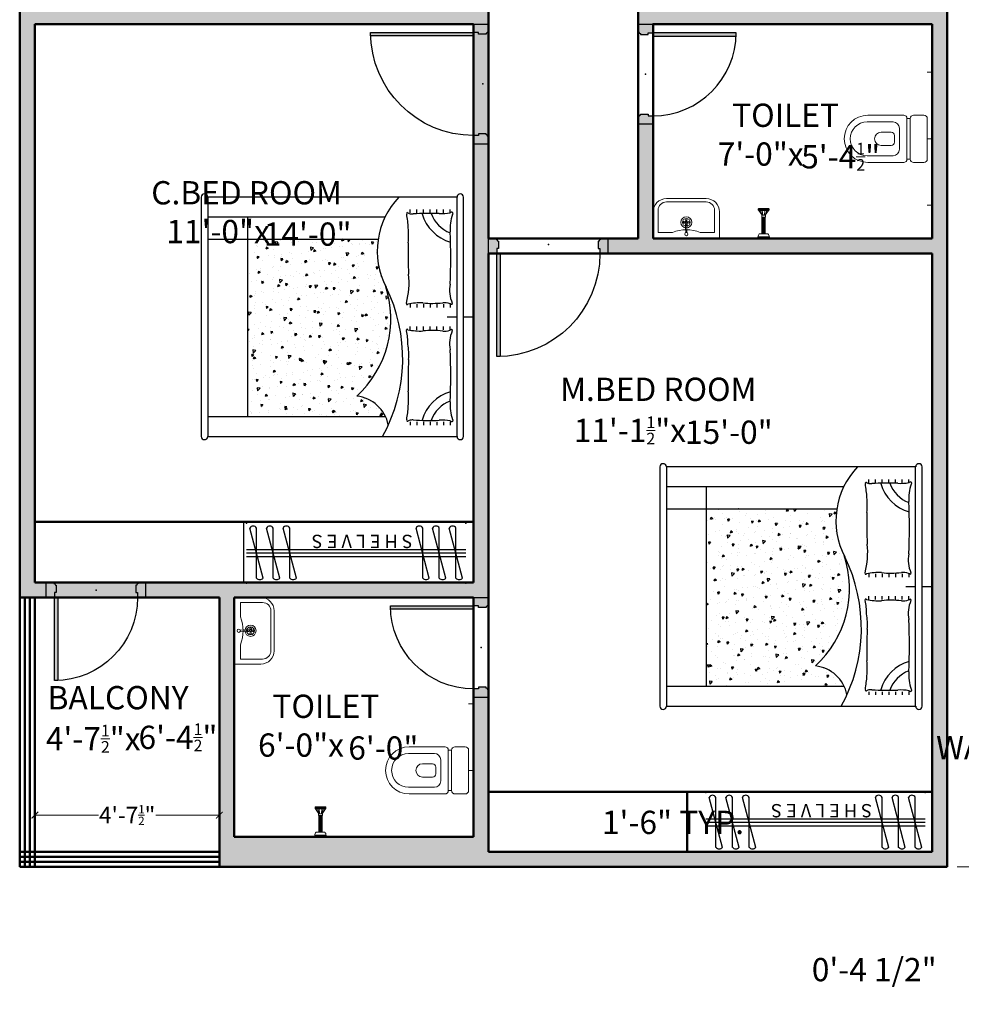
# Model space of a CAD drawing. Units: inches. Extents: x 4508 to 5907, y 877 to 1592.
# Tile 2 of 20: x 4919 to 5203, y 885 to 1182. Entities that reach past the tile are written whole.
import ezdxf

# ---------------------------------------------------------------- set-up
doc = ezdxf.new("R2010")
doc.units = ezdxf.units.IN
doc.layers.get('DEFPOINTS').update_dxf_attribs({"color": 8})
for name, color, linetype, lineweight in [('A-ANNO-DIMS', 2, 'Continuous', 18), ('A-DOOR', 4, 'Continuous', 25), ('A-FLOR-CASE', 30, 'Continuous', 25), ('A-FLOR-FIXT', 8, 'Continuous', 18), ('A-FURN', 24, 'Continuous', 18), ('A-WALL', 7, 'Continuous', 50), ('A-WALL-PATT', 8, 'Continuous', 13)]:
    doc.layers.add(name, color=color, linetype=linetype, lineweight=lineweight)
doc.layers.add('doors & windows', color=30, linetype='Continuous')
doc.layers.add('furniture', color=24, linetype='Continuous')
doc.styles.get("Standard").update_dxf_attribs({"font": 'arial.ttf'})
doc.dimstyles.new('details', dxfattribs={"dimtxt": 5, "dimasz": 2, "dimexe": 2, "dimexo": 3, "dimgap": 1, "dimtad": 0, "dimdec": 1, "dimzin": 0, "dimdsep": 46, "dimlunit": 4, "dimtxsty": 'Standard', "dimblk": 'ARCHTICK', "dimcen": 3, "dimclrd": 256, "dimclre": 256, "dimclrt": 256, "dimadec": 0, "dimazin": 0, "dimtfac": 0.5, "dimtdec": 1, "dimtofl": 0, "dimtmove": 0, "dimatfit": 3, "dimldrblk": 'CLOSEDBLANK', "dimfxl": 2, "dimtolj": 1, "dimtzin": 0, "dimlwd": -1, "dimlwe": -1, "dimarcsym": 0})
doc.dimstyles.new('text', dxfattribs={"dimtxt": 7, "dimasz": 0, "dimexe": 3, "dimexo": 3, "dimgap": 0, "dimtad": 1, "dimtih": 1, "dimtoh": 1, "dimzin": 3, "dimdsep": 46, "dimlunit": 4, "dimtxsty": 'Standard', "dimblk": 'CLOSEDBLANK', "dimcen": 3, "dimse1": 1, "dimse2": 1, "dimsd1": 1, "dimsd2": 1, "dimclrd": 256, "dimclre": 256, "dimclrt": 256, "dimadec": 0, "dimazin": 0, "dimtfac": 0.5, "dimtofl": 0, "dimtmove": 0, "dimatfit": 3, "dimfxl": 3, "dimtolj": 1, "dimtzin": 0, "dimlwd": -1, "dimlwe": -1, "dimarcsym": 0})

# ---------------------------------------------------------------- blocks, each defined once
blk = doc.blocks.new('D2')
at = {"layer": 'doors & windows'}
h = blk.add_hatch(dxfattribs=at)
h.set_pattern_fill('DOTS', color=256, scale=2, angle=180, style=0)
h.set_pattern_definition([(180, (0, -4), (-0.0625, -0.125), [0, -0.125])])
h.paths.add_polyline_path([(2.5, 0), (3.5, 0), (3.5, 24.98, 0.010003), (2.5, 25)])
h = blk.add_hatch(dxfattribs=at)
h.set_pattern_fill('DOTS', color=256, scale=2, angle=180, style=0)
h.set_pattern_definition([(180, (0, 0), (-0.0625, -0.125), [0, -0.125])])
edge = h.paths.add_edge_path()
edge.add_line((27.5, 0), (27.5, -1.5))
edge.add_line((27.5, -1.5), (27, -1.5))
edge.add_line((27, -1.5), (27, -3.75))
edge.add_line((27, -3.75), (27.25, -3.75))
edge.add_arc((27.76, -3.74), 0.509, 181.0059, 268.9941)
edge.add_line((27.75, -4.25), (27.75, -4.5))
edge.add_line((27.75, -4.5), (30, -4.5))
edge.add_line((30, -4.5), (30, 0))
edge.add_line((30, 0), (27.5, 0))
edge = h.paths.add_edge_path()
edge.add_line((2.5, -1.5), (2.5, 0))
edge.add_line((2.5, 0), (0, 0))
edge.add_line((0, 0), (0, -4.5))
edge.add_line((0, -4.5), (2.25, -4.5))
edge.add_line((2.25, -4.5), (2.25, -4.25))
edge.add_arc((2.24, -3.74), 0.509, 271.0059, 358.9941)
edge.add_line((2.75, -3.75), (3, -3.75))
edge.add_line((3, -3.75), (3, -1.5))
edge.add_line((3, -1.5), (2.5, -1.5))
for p, q in [((0, 0), (0, -4.5)), ((30, 0), (30, -4.5))]:
    blk.add_line(p, q)
blk.add_lwpolyline([(3.5, 0), (3.5, 25), (2.5, 25), (2.5, 0)], close=True, dxfattribs=at)
for points in [[(3, -3.75), (3, -1.5), (2.5, -1.5), (2.5, 0), (0, 0)], [(27, -3.75), (27, -1.5), (27.5, -1.5), (27.5, 0), (30, 0)], [(0, -4.5), (2.25, -4.5)], [(30, -4.5), (27.75, -4.5)]]:
    blk.add_lwpolyline(points, dxfattribs=at)
for points in [[(2.25, -4.5), (2.25, -4.25, 0.403966), (2.75, -3.75), (3, -3.75)], [(27.75, -4.5), (27.75, -4.25, -0.403966), (27.25, -3.75), (27, -3.75)]]:
    blk.add_lwpolyline(points, format="xyb", dxfattribs=at)
at = {"layer": 'doors & windows', "ltscale": 6}
blk.add_arc((2.5, 0), 25, 0, 90, dxfattribs=at)
at = {"layer": 'doors & windows'}
blk.add_point((15, -2.25), dxfattribs=at)
blk = doc.blocks.new('*D63')
at = {"layer": 'DEFPOINTS', "color": 0, "transparency": 16777216}
for p in [(5055.99, 966.88), (5055.99, 959.68), (4983.99, 949.27)]:
    blk.add_point(p, dxfattribs=at)
at = {"layer": 'A-ANNO-DIMS', "color": 0, "transparency": 16777216, "insert": (5004.05, 969.15), "char_height": 7, "attachment_point": 5}
blk.add_mtext('\\A1;       TOILET\\P6\'-0"x', dxfattribs=at)
blk = doc.blocks.new('_ClosedBlank')
at = {"color": 0, "lineweight": -2}
for p, q in [((-1, 0.17), (0, 0)), ((-1, 0.17), (-1, -0.17)), ((0, 0), (-1, -0.17))]:
    blk.add_line(p, q, dxfattribs=at)
blk = doc.blocks.new('*D64')
at = {"layer": 'DEFPOINTS', "color": 0, "transparency": 16777216}
for p in [(5016.99, 1007.7), (5023.45, 935.7), (5028.83, 935.7)]:
    blk.add_point(p, dxfattribs=at)
at = {"layer": 'A-ANNO-DIMS', "color": 0, "transparency": 16777216, "insert": (5028.83, 962.43), "char_height": 7, "attachment_point": 5}
blk.add_mtext('\\A1;6\'-0"', dxfattribs=at)
blk = doc.blocks.new('commode')
for p, q in [((-7.09, 19.41), (-7.09, 8.61)), ((-5.09, 11.81), (-5.09, 19.57)), ((5.09, 11.81), (5.09, 19.57)), ((7.09, 19.41), (7.09, 8.61)), ((-2, 12.37), (-2, 15.37)), ((2, 12.37), (2, 15.37)), ((-3.15, 9.87), (3.15, 9.87)), ((-1, 11.37), (1, 11.37)), ((-6.09, 7.61), (6.09, 7.61)), ((-6.09, 6.61), (-6.09, 7.61)), ((-6.09, 6.61), (6.09, 6.61)), ((6.09, 7.61), (6.09, 6.61)), ((-7.09, 2.5), (-7.09, 5.61)), ((7.09, 2.5), (7.09, 5.61)), ((-20, 1.5), (-20, 0)), ((-6.09, 1.5), (6.09, 1.5)), ((0, 1.5), (0, 0)), ((20, 1.5), (20, 0))]:
    blk.add_line(p, q)
for centre, radius, start, end in [((0, 19.41), 7.09, 0, 180), ((0, 19.57), 5.09, 0, 180), ((0, 15.37), 2, 0, 180), ((-1, 12.37), 1, 180, 270), ((1, 12.37), 1, 270, 0), ((-3.15, 11.81), 1.94, 180, 270), ((3.15, 11.81), 1.94, 270, 0), ((-6.09, 8.61), 1, 180, 270), ((-6.09, 5.61), 1, 90, 180), ((6.09, 8.61), 1, 270, 0), ((6.09, 5.61), 1, 0, 90), ((-6.09, 2.5), 1, 180, 270), ((6.09, 2.5), 1, 270, 0)]:
    blk.add_arc(centre, radius, start, end)
blk = doc.blocks.new('wash basin 1')
for p, q in [((0, 10), (-8, 10)), ((0, 10), (0, -10)), ((-12, 6), (-12, -6)), ((-11, 6), (-11, -6)), ((-8.5, 8.5), (-1.85, 8.5)), ((-1.85, 8.5), (-1.85, 4.19)), ((-1.85, -8.5), (-1.85, -4.19)), ((-8.5, -8.5), (-1.85, -8.5)), ((0, -10), (-8, -10))]:
    blk.add_line(p, q)
blk.add_lwpolyline([(-1.83, 0.11), (-5.25, 0.25), (-5.23, -0.38), (-1.8, -0.19)])
for centre, radius in [((-4.87, 0), 1.68), ((-4.87, 0), 1.18), ((-5.63, 0), 0.25), ((-4.87, 0.75), 0.25), ((-4.87, 0), 0.25), ((-4.19, 0), 0.25), ((-1.34, 0), 0.5), ((-4.87, -0.72), 0.25)]:
    blk.add_circle(centre, radius)
for centre, radius, start, end in [((-8, 6), 4, 90, 180), ((-8.5, 6), 2.5, 90, 180), ((8.89, 0), 11.53, 158.7059, 201.2941), ((-8, -6), 4, 180, 270), ((-8.5, -6), 2.5, 180, 270)]:
    blk.add_arc(centre, radius, start, end)
blk = doc.blocks.new('tap & shower')
for p, q in [((1.71, 0), (-1.71, 0)), ((-1.71, 0), (-1.71, -0.5)), ((1.71, 0), (1.71, -0.5)), ((1.71, -0.5), (-1.71, -0.5)), ((1.31, -1.4), (-1.31, -1.4)), ((-0.5, -6.44), (-0.5, -1.4)), ((-0.42, -6.44), (-0.42, -1.4)), ((-0.32, -0.5), (0.32, -0.5)), ((-0.3, -6.44), (-0.3, -1.4)), ((-0.14, -6.44), (-0.14, -1.4)), ((0.14, -6.44), (0.14, -1.4)), ((0.3, -6.44), (0.3, -1.4)), ((0.42, -6.44), (0.42, -1.4)), ((0.5, -6.44), (0.5, -1.4)), ((-1.62, -8.87), (-1.62, -8.6)), ((-1.48, -8.46), (-0.47, -6.98)), ((-1.48, -8.46), (1.48, -8.46)), ((-1.48, -9), (-1.48, -8.46)), ((-1.43, -9), (-1.43, -8.46)), ((-1.37, -9), (-1.37, -8.46)), ((-1.32, -9), (-1.32, -8.46)), ((-1.27, -9), (-1.27, -8.46)), ((-1.21, -9), (-1.21, -8.46)), ((-1.16, -9), (-1.16, -8.46)), ((-1.1, -9), (-1.1, -8.46)), ((-1.05, -9), (-1.05, -8.46)), ((-1, -9), (-1, -8.46)), ((-0.41, -6.98), (-0.94, -8.46)), ((-0.94, -9), (-0.94, -8.46)), ((-0.89, -9), (-0.89, -8.46)), ((-0.84, -9), (-0.84, -8.46)), ((-0.78, -9), (-0.78, -8.46)), ((-0.73, -9), (-0.73, -8.46)), ((-0.67, -9), (-0.67, -8.46)), ((-0.62, -9), (-0.62, -8.46)), ((-0.57, -9), (-0.57, -8.46)), ((-0.56, -6.44), (0.56, -6.44)), ((-0.56, -6.98), (-0.56, -6.44)), ((-0.56, -6.98), (0.56, -6.98)), ((-0.51, -9), (-0.51, -8.46)), ((-0.46, -9), (-0.46, -8.46)), ((-0.29, -6.98), (-0.4, -8.46)), ((-0.4, -9), (-0.4, -8.46)), ((-0.35, -9), (-0.35, -8.46)), ((-0.3, -9), (-0.3, -8.46)), ((-0.24, -9), (-0.24, -8.46)), ((-0.19, -9), (-0.19, -8.46)), ((-0.13, -9), (-0.13, -8.46)), ((-0.08, -9), (-0.08, -8.46)), ((-0.03, -9), (-0.03, -8.46)), ((0.03, -9), (0.03, -8.46)), ((0.08, -9), (0.08, -8.46)), ((0.13, -9), (0.13, -8.46)), ((0.19, -9), (0.19, -8.46)), ((0.24, -9), (0.24, -8.46)), ((0.29, -6.98), (0.4, -8.46)), ((0.3, -9), (0.3, -8.46)), ((0.35, -9), (0.35, -8.46)), ((0.4, -9), (0.4, -8.46)), ((0.41, -6.98), (0.94, -8.46)), ((0.46, -9), (0.46, -8.46)), ((1.48, -8.46), (0.47, -6.98)), ((0.51, -9), (0.51, -8.46)), ((0.56, -6.98), (0.56, -6.44)), ((0.57, -9), (0.57, -8.46)), ((0.62, -9), (0.62, -8.46)), ((0.67, -9), (0.67, -8.46)), ((0.73, -9), (0.73, -8.46)), ((0.78, -9), (0.78, -8.46)), ((0.84, -9), (0.84, -8.46)), ((0.89, -9), (0.89, -8.46)), ((0.94, -9), (0.94, -8.46)), ((1, -9), (1, -8.46)), ((1.05, -9), (1.05, -8.46)), ((1.1, -9), (1.1, -8.46)), ((1.16, -9), (1.16, -8.46)), ((1.21, -9), (1.21, -8.46)), ((1.27, -9), (1.27, -8.46)), ((1.32, -9), (1.32, -8.46)), ((1.37, -9), (1.37, -8.46)), ((1.43, -9), (1.43, -8.46)), ((1.48, -9), (1.48, -8.46)), ((1.62, -8.87), (1.62, -8.6)), ((-1.48, -9), (1.48, -9))]:
    blk.add_line(p, q)
for centre, radius, start, end in [((-0.02, -0.29), 1.7, 187.1825, 220.9028), ((0.02, -0.29), 1.7, 319.0972, 352.8175), ((-1.48, -8.6), 0.135, 90, 180), ((-1.48, -8.87), 0.135, 180, 270), ((1.48, -8.6), 0.135, 0, 90), ((1.48, -8.87), 0.135, 270, 0)]:
    blk.add_arc(centre, radius, start, end)
blk = doc.blocks.new('*D65')
at = {"layer": 'DEFPOINTS', "color": 0, "transparency": 16777216}
for p in [(4979.49, 965.56), (4923.99, 960.73), (4979.49, 961.06)]:
    blk.add_point(p, dxfattribs=at)
at = {"layer": 'A-ANNO-DIMS', "color": 0, "transparency": 16777216, "insert": (4941.54, 971.05), "char_height": 7, "attachment_point": 5}
blk.add_mtext('\\A1;       BALCONY\\P4\'-7{\\H0.5x;\\S1/2;}"x', dxfattribs=at)
blk = doc.blocks.new('*D66')
at = {"layer": 'DEFPOINTS', "color": 0, "transparency": 16777216}
for p in [(4957.4, 1007.7), (4953.38, 931.2), (4967.04, 931.2)]:
    blk.add_point(p, dxfattribs=at)
at = {"layer": 'A-ANNO-DIMS', "color": 0, "transparency": 16777216, "insert": (4967.04, 965.63), "char_height": 7, "attachment_point": 5}
blk.add_mtext('\\A1;6\'-4{\\H0.5x;\\S1/2;}"', dxfattribs=at)
blk = doc.blocks.new('*D67')
at = {"layer": 'DEFPOINTS', "color": 0, "transparency": 16777216}
for p in [(5139.49, 1111.2), (5132.79, 931.2), (5134.28, 931.2)]:
    blk.add_point(p, dxfattribs=at)
at = {"layer": 'A-ANNO-DIMS', "color": 0, "transparency": 16777216, "insert": (5132.79, 1057.44), "char_height": 7, "attachment_point": 5}
blk.add_mtext('\\A1;15\'-0"', dxfattribs=at)
blk = doc.blocks.new('*D68')
at = {"layer": 'DEFPOINTS', "color": 0, "transparency": 16777216}
for p in [(5193.99, 1053.82), (5060.49, 1032.61), (5193.99, 1023.97)]:
    blk.add_point(p, dxfattribs=at)
at = {"layer": 'A-ANNO-DIMS', "color": 0, "transparency": 16777216, "insert": (5103.01, 1063.81), "char_height": 7, "attachment_point": 5}
blk.add_mtext('\\A1;        M.BED ROOM\\P11\'-1{\\H0.5x;\\S1/2;}"x', dxfattribs=at)
blk = doc.blocks.new('bed')
at = {"layer": 'furniture'}
h = blk.add_hatch(dxfattribs=at)
h.set_pattern_fill('AR-CONC', color=256, angle=-90, style=0)
h.set_pattern_definition([(320, (0, 2.38), (-0.6275, -7.1726), [0.75, -8.25]), (265, (0, 2.38), (7.5219, 1.3875), [0.6, -6.6]), (10.451, (-0.052, 1.782), (6.8944, -5.7851), [0.6374, -7.0114]), (316.184, (2, 2.38), (-1.6552, -10.6724), [1.125, -12.375]), (6.636, (1.862, 1.491), (9.7412, -9.3466), [0.9561, -10.5171]), (261.184, (2, 2.38), (9.7412, -9.3466), [0.9, -9.9]), (291, (1.5, 1.38), (-4.0262, -5.96907), [0.75, -8.25]), (236, (1.5, 1.38), (7.2515, -2.43315), [0.6, -6.6]), (341.451, (1.1645, 0.8826), (3.2253, -8.4022), [0.6374, -7.0114]), (307.5, (0, 2.38), (3.32894, -0.1216), [0, -6.52, 0, -6.7, 0, -6.625]), (277.5, (0, 2.38), (3.94412, -2.6307), [0, -3.82, 0, -6.37, 0, -2.525]), (237.5, (0, 4.61), (-0.22555, -5.33822), [0, -2.5, 0, -7.8, 0, -10.35]), (227.5, (0, 5.61), (1.00105, -5.83186), [0, -3.25, 0, -5.18, 0, -7.35])])
h.paths.add_polyline_path([(30.01, -68), (30.01, -26.5, 0.263043), (23.9, -35.15, 0.293424), (-9.18, -26.47, -0.156683), (-23.39, -28.72), (-23.39, -68)])
for p, q in [((0, -3), (0, 0)), ((36.01, -3), (-36.01, -3)), ((-36.01, -5), (-36.01, -80)), ((36.01, -5), (-36.01, -5)), ((0, -8), (0, -5)), ((36.01, -80), (36.01, -5)), ((-31.24, -7.07), (-32.24, -7.07)), ((-3.81, -7.07), (-2.81, -7.07)), ((3.89, -7.07), (2.89, -7.07)), ((31.63, -7.07), (32.63, -7.07)), ((-31.24, -9.07), (-32.24, -9.07)), ((-31.24, -11.07), (-32.24, -11.07)), ((-3.81, -9.07), (-2.81, -9.07)), ((-3.81, -11.07), (-2.81, -11.07)), ((3.89, -9.07), (2.89, -9.07)), ((3.89, -11.07), (2.89, -11.07)), ((31.63, -9.07), (32.63, -9.07)), ((31.63, -11.07), (32.63, -11.07)), ((-31.24, -13.07), (-32.24, -13.07)), ((-3.81, -13.07), (-2.81, -13.07)), ((3.89, -13.07), (2.89, -13.07)), ((31.63, -13.07), (32.63, -13.07)), ((-31.24, -15.07), (-32.24, -15.07)), ((-31.24, -17.07), (-32.24, -17.07)), ((-3.81, -15.07), (-2.81, -15.07)), ((-3.81, -17.07), (-2.81, -17.07)), ((3.89, -15.07), (2.89, -15.07)), ((3.89, -17.07), (2.89, -17.07)), ((31.63, -15.07), (32.63, -15.07)), ((31.63, -17.07), (32.63, -17.07)), ((-31.24, -19.07), (-32.24, -19.07)), ((-3.81, -19.07), (-2.81, -19.07)), ((3.89, -19.07), (2.89, -19.07)), ((31.63, -19.07), (32.63, -19.07)), ((-36.01, -80), (36.01, -80)), ((-36.01, -82), (36.01, -82))]:
    blk.add_line(p, q, dxfattribs=at)
at = {"layer": 'furniture', "ltscale": 7}
blk.add_line((30.01, -80), (30.01, -26.5), dxfattribs=at)
at = {"layer": 'furniture', "ltscale": 5}
blk.add_line((-30.01, -26.66), (-30.01, -80), dxfattribs=at)
at = {"layer": 'furniture', "ltscale": 0.3}
for p, q in [((-23.39, -80), (-23.39, -28.72)), ((-30.01, -68), (30.01, -68))]:
    blk.add_line(p, q, dxfattribs=at)
at = {"layer": 'furniture'}
for centre, radius, start, end in [((-35.95, -4), 1, 93.3831, 266.6169), ((35.95, -4), 1, 273.3831, 86.6169), ((-31.1, -6.57), 0.382, 35.8976, 208.6272), ((-44.44, -13.85), 14.82, 27.1629, 28.6272), ((-46.76, -9.65), 15.72, 357.4804, 9.3956), ((-34.45, -3.51), 9.85, 289.8695, 338.9843), ((-34.45, -3.51), 12.47, 286.0319, 344.1205), ((-26.35, 6.68), 13.76, 251.1782, 273.3982), ((-18.02, -163.6), 156.72, 87.0032, 92.7497), ((-8.03, 2.03), 9.29, 258.896, 294.7184), ((0.25, -8.8), 4.49, 159.0146, 186.273), ((-4.03, -6.67), 0.282, 335.7259, 114.303), ((3.22, -9.94), 7.68, 155.7259, 159.0146), ((4.11, -6.67), 0.282, 65.697, 204.2741), ((-3.14, -9.94), 7.68, 20.9854, 24.2741), ((-0.17, -8.8), 4.49, 353.727, 20.9854), ((8.12, 2.03), 9.29, 245.2816, 281.104), ((18.1, -163.6), 156.72, 87.2503, 92.9968), ((34.54, -3.51), 12.47, 195.8795, 253.9681), ((34.54, -3.51), 9.85, 201.0157, 250.1305), ((26.43, 6.68), 13.76, 266.6018, 288.8218), ((31.18, -6.57), 0.382, 331.3728, 144.1024), ((46.84, -9.65), 15.72, 170.6044, 182.5196), ((44.53, -13.85), 14.82, 151.3728, 152.8371), ((-28.62, 31.03), 42.31, 266.4836, 266.6487), ((54.88, -13.16), 85.99, 178.1209, 183.3613), ((-32.82, -12.44), 28.78, 354.3784, 6.273), ((32.9, -12.44), 28.78, 173.727, 185.6216), ((-54.8, -13.16), 85.99, 356.6387, 1.8791), ((28.7, 31.03), 42.31, 273.3513, 273.5164), ((12.28, -16.11), 16.48, 177.0317, 192.8678), ((-12.19, -16.11), 16.48, 347.1322, 2.9683), ((-31.05, -19.91), 0.291, 147.6219, 311.9343), ((-33.2, -18.55), 2.25, 327.6219, 339.2246), ((-34.13, -18.41), 3.18, 342.7809, 3.755), ((-24.4, -58.01), 38.42, 93.5164, 99.6766), ((-24.52, -56.06), 36.48, 86.4836, 93.5164), ((-18.49, 70.49), 90.23, 267.5921, 273.6329), ((-10.31, -44.95), 25.52, 75.952, 95.5452), ((-3.95, -19.99), 0.265, 231.9005, 52.8902), ((4.03, -19.99), 0.265, 127.1098, 308.0995), ((7.57, -34.68), 14.87, 87.3976, 103.1191), ((11.44, -34.81), 15.32, 84.694, 102.0355), ((18.57, 70.49), 90.23, 266.3671, 272.4079), ((24.6, -56.06), 36.48, 86.4836, 93.5164), ((24.48, -58.01), 38.42, 80.3234, 86.4836), ((31.13, -19.91), 0.291, 228.0657, 32.3781), ((34.21, -18.41), 3.18, 176.245, 197.2191), ((33.28, -18.55), 2.25, 200.7754, 212.3781), ((-19.79, -5.47), 23.53, 226.4061, 297.4441), ((12.51, -69.71), 48.38, 60.9345, 116.3227), ((0.6, -56.57), 31.65, 42.5874, 108.5034), ((34.61, -36.23), 10.76, 101.1719, 174.259), ((-35.95, -81), 1, 93.3831, 266.6169), ((35.95, -81), 1, 273.3831, 86.6169)]:
    blk.add_arc(centre, radius, start, end, dxfattribs=at)
blk = doc.blocks.new('hangers')
at = {"layer": 'furniture'}
for p, q in [((1, 7.5), (5, -7.5)), ((3, 7.5), (3, -7.5)), ((6, 7.5), (10, -7.5)), ((8, 7.5), (8, -7.5)), ((11, 7.5), (15, -7.5)), ((13, 7.5), (13, -7.5)), ((51, 7.5), (55, -7.5)), ((53, 7.5), (53, -7.5)), ((56, 7.5), (60, -7.5)), ((58, 7.5), (58, -7.5)), ((61, 7.5), (65, -7.5)), ((63, 7.5), (63, -7.5)), ((66, 1), (0, 1)), ((0, 0), (66, 0)), ((0, -1), (66, -1))]:
    blk.add_line(p, q, dxfattribs=at)
for centre, radius, start, end in [((2, 6.62), 1.33, 41.2884, 138.7116), ((7, 6.62), 1.33, 41.2884, 138.7116), ((12, 6.62), 1.33, 41.2884, 138.7116), ((52, 6.62), 1.33, 41.2884, 138.7116), ((57, 6.62), 1.33, 41.2884, 138.7116), ((62, 6.62), 1.33, 41.2884, 138.7116), ((4, -7.08), 1.08, 202.5549, 337.4451), ((9, -7.08), 1.08, 202.5549, 337.4451), ((14, -7.08), 1.08, 202.5549, 337.4451), ((54, -7.08), 1.08, 202.5549, 337.4451), ((59, -7.08), 1.08, 202.5549, 337.4451), ((64, -7.08), 1.08, 202.5549, 337.4451)]:
    blk.add_arc(centre, radius, start, end, dxfattribs=at)
for p in [(0, 9), (66, 9), (0, -9), (66, -9)]:
    blk.add_point(p, dxfattribs=at)
blk.add_text('S H E L V E S', height=4, dxfattribs=at).set_placement((16, -5.52))
blk = doc.blocks.new('D1')
at = {"layer": 'doors & windows'}
h = blk.add_hatch(dxfattribs=at)
h.set_pattern_fill('DOTS', color=256, scale=2, angle=180, style=0)
h.set_pattern_definition([(180, (-2e-12, -4), (-0.0625, -0.125), [0, -0.125])])
h.paths.add_polyline_path([(2.5, 0), (3.5, 0), (3.5, 30.98, 0.008066), (2.5, 31)])
h = blk.add_hatch(dxfattribs=at)
h.set_pattern_fill('DOTS', color=256, scale=2, angle=180, style=0)
h.set_pattern_definition([(180, (0, -0.5), (-0.0625, -0.125), [0, -0.125])])
h.paths.add_polyline_path([(0, -4.5), (2.25, -4.5), (2.25, -4.25, 0.403966), (2.75, -3.75), (3, -3.75), (3, -1.5), (2.5, -1.5), (2.5, 0), (0, 0)])
h.paths.add_polyline_path([(36, -4.5), (36, 0), (33.5, 0), (33.5, -1.5), (33, -1.5), (33, -3.75), (33.25, -3.75, 0.403966), (33.75, -4.25), (33.75, -4.5)])
for p, q in [((0, 0), (0, -4.5)), ((36, 0), (36, -4.5))]:
    blk.add_line(p, q)
blk.add_lwpolyline([(3.5, 0), (3.5, 31), (2.5, 31), (2.5, 0)], close=True, dxfattribs=at)
for points in [[(3, -3.75), (3, -1.5), (2.5, -1.5), (2.5, 0), (0, 0)], [(33, -3.75), (33, -1.5), (33.5, -1.5), (33.5, 0), (36, 0)], [(0, -4.5), (2.25, -4.5)], [(36, -4.5), (33.75, -4.5)]]:
    blk.add_lwpolyline(points, dxfattribs=at)
for points in [[(2.25, -4.5), (2.25, -4.25, 0.403966), (2.75, -3.75), (3, -3.75)], [(33.75, -4.5), (33.75, -4.25, -0.403966), (33.25, -3.75), (33, -3.75)]]:
    blk.add_lwpolyline(points, format="xyb", dxfattribs=at)
at = {"layer": 'doors & windows', "ltscale": 6}
blk.add_arc((2.5, 0), 31, 0, 90, dxfattribs=at)
at = {"layer": 'doors & windows'}
blk.add_point((18, -2.75), dxfattribs=at)
blk = doc.blocks.new('*D69')
at = {"layer": 'DEFPOINTS', "color": 0, "transparency": 16777216}
for p in [(4989.99, 1180.2), (5002.84, 1012.2), (5006.05, 1012.2)]:
    blk.add_point(p, dxfattribs=at)
at = {"layer": 'A-ANNO-DIMS', "color": 0, "transparency": 16777216, "insert": (5006.05, 1117.03), "char_height": 7, "attachment_point": 5}
blk.add_mtext('\\A1;14\'-0"', dxfattribs=at)
blk = doc.blocks.new('*D70')
at = {"layer": 'DEFPOINTS', "color": 0, "transparency": 16777216}
for p in [(5055.99, 1128.18), (4923.99, 1122.54), (5055.99, 1114.17)]:
    blk.add_point(p, dxfattribs=at)
at = {"layer": 'A-ANNO-DIMS', "color": 0, "transparency": 16777216, "insert": (4979.11, 1123.64), "char_height": 7, "attachment_point": 5}
blk.add_mtext('\\A1;        C.BED ROOM\\P11\'-0"x', dxfattribs=at)
blk = doc.blocks.new('*D73')
at = {"layer": 'DEFPOINTS', "color": 0, "transparency": 16777216}
for p in [(5193.99, 1151.7), (5193.99, 1137.48), (5109.99, 1130.02)]:
    blk.add_point(p, dxfattribs=at)
at = {"layer": 'A-ANNO-DIMS', "color": 0, "transparency": 16777216, "insert": (5142.36, 1146.95), "char_height": 7, "attachment_point": 5}
blk.add_mtext('\\A1;       TOILET\\P7\'-0"x', dxfattribs=at)
blk = doc.blocks.new('*D74')
at = {"layer": 'DEFPOINTS', "color": 0, "transparency": 16777216}
for p in [(5156.68, 1180.2), (5156.68, 1115.7), (5166.43, 1115.7)]:
    blk.add_point(p, dxfattribs=at)
at = {"layer": 'A-ANNO-DIMS', "color": 0, "transparency": 16777216, "insert": (5166.43, 1140.3), "char_height": 7, "attachment_point": 5}
blk.add_mtext('\\A1;5\'-4{\\H0.5x;\\S1/2;}"', dxfattribs=at)
blk = doc.blocks.new('_ArchTick')
at = {"color": 0, "linetype": 'ByBlock', "const_width": 0.15}
blk.add_lwpolyline([(-0.5, -0.5), (0.5, 0.5)], dxfattribs=at)
blk = doc.blocks.new('*D77')
at = {"layer": 'A-ANNO-DIMS', "color": 0, "transparency": 16777216}
for p, q in [((5201.49, 1574.7), (5213.97, 1574.7)), ((5211.97, 1574.7), (5211.97, 1255.95)), ((5211.97, 926.7), (5211.97, 1245.46)), ((5201.49, 926.7), (5213.97, 926.7))]:
    blk.add_line(p, q, dxfattribs=at)
at = {"layer": 'DEFPOINTS', "color": 0, "transparency": 16777216}
for p in [(5198.49, 1574.7), (5211.97, 1574.7), (5198.49, 926.7)]:
    blk.add_point(p, dxfattribs=at)
at = {"layer": 'A-ANNO-DIMS', "color": 0, "transparency": 16777216, "xscale": 2, "yscale": 2, "zscale": 2}
for p, rotation in [((5211.97, 1574.7), 90), ((5211.97, 926.7), 270)]:
    blk.add_blockref('_ArchTick', p, dxfattribs=dict(at, rotation=rotation))
at = {"layer": 'A-ANNO-DIMS', "color": 0, "transparency": 16777216, "insert": (5211.97, 1250.7), "char_height": 5, "attachment_point": 5, "rotation": 90}
blk.add_mtext("\\A1;54'", dxfattribs=at)
blk = doc.blocks.new('*D102')
at = {"layer": 'A-ANNO-DIMS', "color": 0, "transparency": 16777216}
for p, q in [((4923.99, 934.2), (4923.99, 944.26)), ((4923.99, 942.26), (4943.08, 942.26)), ((4979.49, 942.26), (4960.4, 942.26)), ((4979.49, 934.2), (4979.49, 944.26))]:
    blk.add_line(p, q, dxfattribs=at)
at = {"layer": 'DEFPOINTS', "color": 0, "transparency": 16777216}
for p in [(4979.49, 942.26), (4923.99, 931.2), (4979.49, 931.2)]:
    blk.add_point(p, dxfattribs=at)
at = {"layer": 'A-ANNO-DIMS', "color": 0, "transparency": 16777216, "xscale": 2, "yscale": 2, "zscale": 2, "rotation": 180}
blk.add_blockref('_ArchTick', (4923.99, 942.26), dxfattribs=at)
at = {"layer": 'A-ANNO-DIMS', "color": 0, "transparency": 16777216, "xscale": 2, "yscale": 2, "zscale": 2}
blk.add_blockref('_ArchTick', (4979.49, 942.26), dxfattribs=at)
at = {"layer": 'A-ANNO-DIMS', "color": 0, "transparency": 16777216, "insert": (4951.74, 942.26), "char_height": 5, "attachment_point": 5}
blk.add_mtext('\\A1;4\'-7{\\H0.5x;\\S1/2;}"', dxfattribs=at)
blk = doc.blocks.new('*D156')
at = {"layer": 'DEFPOINTS', "color": 0, "transparency": 16777216}
for p in [(5125.87, 958.96), (5125.87, 949.06), (5191.87, 949.06)]:
    blk.add_point(p, dxfattribs=at)
at = {"layer": 'A-ANNO-DIMS', "transparency": 16777216, "insert": (5243.5, 962.58), "char_height": 7, "attachment_point": 5}
blk.add_mtext('\\A1;WARDROBE 5\'-6" TYP.', dxfattribs=at)
blk = doc.blocks.new('*D157')
at = {"layer": 'DEFPOINTS', "color": 0, "transparency": 16777216}
for p in [(5125.87, 949.06), (5115.97, 931.06), (5125.87, 931.06)]:
    blk.add_point(p, dxfattribs=at)
at = {"layer": 'A-ANNO-DIMS', "transparency": 16777216, "insert": (5115.97, 940.06), "char_height": 7, "attachment_point": 5}
blk.add_mtext('\\A1;1\'-6" TYP.', dxfattribs=at)
blk = doc.blocks.new('*D186')
at = {"layer": 'DEFPOINTS', "color": 0, "transparency": 16777216}
for p in [(5193.99, 931.2), (5198.49, 926.7), (5198.49, 892.15)]:
    blk.add_point(p, dxfattribs=at)
at = {"layer": 'A-ANNO-DIMS', "transparency": 16777216, "insert": (5176.53, 895.77), "char_height": 7, "attachment_point": 5}
blk.add_mtext('\\A1;0\'-4 1/2"', dxfattribs=at)
blk = doc.blocks.new('*D187')
at = {"layer": 'DEFPOINTS', "color": 0, "transparency": 16777216}
for p in [(4884.94, 1184.7), (4923.99, 1184.7), (4923.99, 1180.2)]:
    blk.add_point(p, dxfattribs=at)
at = {"layer": 'A-ANNO-DIMS', "transparency": 16777216, "insert": (4902.4, 1183.82), "char_height": 7, "attachment_point": 5}
blk.add_mtext('\\A1;0\'-4 1/2"', dxfattribs=at)

msp = doc.modelspace()

# ---------------------------------------------------------------- hatches: boundary and pattern name
at = {"layer": 'A-WALL-PATT'}
h = msp.add_hatch(color=256, dxfattribs=at)
h.dxf.hatch_style = 1
h.paths.add_polyline_path([(5198.492, 1328.704), (5148.992, 1328.704), (5148.992, 1340.919), (5144.492, 1340.919), (5144.492, 1328.704), (5130.194, 1328.704), (5130.194, 1324.204), (5163.992, 1324.204), (5163.992, 1184.704), (5105.492, 1184.704), (5105.492, 1180.124), (5109.992, 1180.124), (5109.992, 1180.204), (5193.992, 1180.204), (5193.992, 1115.704), (5109.992, 1115.704), (5109.992, 1123.704), (5109.992, 1150.124), (5105.492, 1150.124), (5105.492, 1115.704), (5096.492, 1115.704), (5096.492, 1111.204), (5193.992, 1111.204), (5193.992, 931.204), (5060.492, 931.204), (5060.492, 977.704), (5055.992, 977.704), (5055.992, 935.704), (5054.492, 935.704), (4983.992, 935.704), (4983.992, 1007.704), (4991.992, 1007.704), (5055.992, 1007.704), (5060.492, 1007.704), (5060.492, 1111.204), (5060.492, 1115.704), (5060.492, 1144.204), (5055.992, 1144.204), (5055.992, 1012.204), (4957.397, 1012.204), (4957.397, 1007.704), (4979.492, 1007.704), (4979.492, 926.704), (5198.492, 926.704)])
h.paths.add_polyline_path([(5193.992, 1184.704), (5168.492, 1184.704), (5168.492, 1324.204), (5193.992, 1324.204)], flags=16)
h.paths.add_polyline_path([(4923.992, 1180.204), (5055.992, 1180.204), (5055.992, 1144.204), (5060.492, 1144.204), (5060.492, 1184.704), (4923.992, 1184.704), (4923.992, 1424.704), (4923.992, 1433.704), (4919.492, 1433.704), (4919.492, 1007.704), (4957.397, 1007.704), (4957.397, 1012.204), (4923.992, 1012.204)])

# ---------------------------------------------------------------- linework, layer by layer
at = {"layer": 'A-FLOR-CASE'}
for p, q in [((4986.727, 1030.513), (4986.727, 1012.204)), ((5060.492, 1030.513), (5060.518, 1030.513))]:
    msp.add_line(p, q, dxfattribs=at)
at = {"layer": 'A-WALL'}
for p, q in [((4919.492, 926.704), (4919.492, 1574.704)), ((5198.492, 1574.704), (5198.492, 926.704)), ((5060.492, 1184.704), (5060.492, 1115.704)), ((4923.992, 1012.204), (4923.992, 1180.204)), ((5055.992, 1012.204), (5055.992, 1180.204)), ((5193.992, 1180.204), (5193.992, 1115.704)), ((5105.492, 1115.704), (5060.492, 1115.704)), ((5193.992, 1115.704), (5109.992, 1115.704)), ((5193.992, 1111.204), (5060.492, 1111.204)), ((5060.492, 1111.204), (5060.492, 931.204)), ((5193.992, 1111.204), (5193.992, 931.204)), ((4923.992, 1030.513), (5055.992, 1030.513)), ((4979.492, 1007.704), (4919.492, 1007.704)), ((4920.992, 926.704), (4920.992, 1007.704)), ((4922.492, 926.704), (4922.492, 1007.704)), ((4923.992, 926.704), (4923.992, 1007.704)), ((4979.492, 926.704), (4979.492, 1007.704)), ((5055.992, 1007.704), (4983.992, 1007.704)), ((4983.992, 935.704), (4983.992, 1007.704)), ((5055.992, 935.704), (5055.992, 1007.704)), ((5060.492, 949.204), (5193.992, 949.204)), ((5120.201, 949.204), (5120.201, 931.204)), ((5055.992, 935.704), (4983.992, 935.704)), ((4979.492, 931.204), (4919.492, 931.204)), ((5193.992, 931.204), (5060.492, 931.204)), ((4979.492, 929.704), (4919.492, 929.704)), ((4979.492, 928.204), (4919.492, 928.204)), ((5198.492, 926.704), (4919.492, 926.704))]:
    msp.add_line(p, q, dxfattribs=at)
for points in [[(5105.492, 1115.704), (5105.492, 1184.704), (5163.992, 1184.704)], [(4923.992, 1180.204), (5055.992, 1180.204)], [(5109.992, 1115.704), (5109.992, 1180.204), (5193.992, 1180.204)], [(4923.992, 1012.204), (5055.992, 1012.204)]]:
    msp.add_lwpolyline(points, dxfattribs=at)

# ---------------------------------------------------------------- block references
at = {"layer": 'A-DOOR', "xscale": -1}
for name, p, rotation in [('D1', (5055.992, 1180.204), 90.0000000000116), ('D1', (5060.492, 1111.204), 180), ('D2', (4927.397, 1007.704), 180), ('D2', (5055.992, 1007.704), 90)]:
    msp.add_blockref(name, p, dxfattribs=dict(at, rotation=rotation))
at = {"layer": 'A-DOOR', "rotation": 270}
msp.add_blockref('D2', (5109.992, 1180.124), dxfattribs=at)
at = {"layer": 'A-FLOR-FIXT'}
for name, p, rotation in [('commode', (5193.992, 1145.704), 90), ('wash basin 1', (5119.992, 1115.704), 270), ('wash basin 1', (4983.992, 997.704), 180)]:
    msp.add_blockref(name, p, dxfattribs=dict(at, rotation=rotation))
at = {"layer": 'A-FLOR-FIXT', "xscale": -1}
for name, p, rotation in [('tap & shower', (5143.255, 1115.704), 180), ('commode', (5055.992, 955.704), 90), ('tap & shower', (5009.917, 935.704), 180)]:
    msp.add_blockref(name, p, dxfattribs=dict(at, rotation=rotation))
at = {"layer": 'A-FURN'}
for name, p, rotation in [('bed', (5055.992, 1092.162), 270), ('bed', (5193.992, 1011.014), 270), ('hangers', (5053.664, 1021.056), 180), ('hangers', (5191.873, 940.056), 180)]:
    msp.add_blockref(name, p, dxfattribs=dict(at, rotation=rotation))

# ---------------------------------------------------------------- dimensions: what is measured, and where the dimension line sits
at = {"layer": 'A-ANNO-DIMS'}
for base, p1, p2, dimstyle, override, picture, middle in [((5211.971, 1574.704), (5198.492, 926.704), (5198.492, 1574.704), 'details', {"dimclrd": 0, "dimclre": 0, "dimclrt": 0}, '*D77', (5211.971, 1250.704)), ((4884.942, 1184.704), (4923.992, 1180.204), (4923.992, 1184.704), 'text', {"dimdec": 1, "dimlfac": 1, "dimrnd": 0, "dimzin": 1, "dimdsep": 46, "dimlunit": 4, "dimfrac": 2}, '*D187', (4902.401, 1183.823))]:
    dim = msp.add_linear_dim(base=base, p1=p1, p2=p2, angle=90, dimstyle=dimstyle, override=override, dxfattribs=at)
    dim.commit()
    dim.dimension.update_dxf_attribs({"geometry": picture, "text_midpoint": middle})
for base, p1, p2, picture, middle in [((5006.051, 1012.204), (4989.992, 1180.204), (5002.845, 1012.204), '*D69', (5006.051, 1117.033)), ((5166.425, 1115.704), (5156.678, 1180.204), (5156.678, 1115.704), '*D74', (5166.425, 1140.301)), ((5132.793, 931.204), (5139.489, 1111.204), (5134.282, 931.204), '*D67', (5132.793, 1057.439)), ((4967.044, 931.204), (4957.397, 1007.704), (4953.375, 931.204), '*D66', (4967.044, 965.635)), ((5028.834, 935.704), (5016.992, 1007.704), (5023.451, 935.704), '*D64', (5028.834, 962.433))]:
    dim = msp.add_linear_dim(base=base, p1=p1, p2=p2, angle=90, dimstyle='text', override={"dimclrd": 0, "dimclre": 0, "dimclrt": 0}, dxfattribs=at)
    dim.commit()
    dim.dimension.update_dxf_attribs({"geometry": picture, "text_midpoint": middle, "dimtype": 160})
for base, p1, p2, text, picture, middle in [((5193.992, 1137.479), (5109.992, 1130.02), (5193.992, 1151.704), '       TOILET\\P<>x', '*D73', (5142.361, 1137.479)), ((5055.992, 1114.173), (4923.992, 1122.538), (5055.992, 1128.18), '        C.BED ROOM\\P<>x', '*D70', (4979.111, 1114.173)), ((5193.992, 1053.819), (5060.492, 1032.61), (5193.992, 1023.969), '        M.BED ROOM\\P<>x', '*D68', (5103.015, 1053.819)), ((4979.492, 961.055), (4923.992, 960.73), (4979.492, 965.557), '       BALCONY\\P<>x', '*D65', (4941.545, 961.055)), ((5055.992, 959.677), (4983.992, 949.275), (5055.992, 966.881), '       TOILET\\P<>x', '*D63', (5004.053, 959.677))]:
    dim = msp.add_linear_dim(base=base, p1=p1, p2=p2, text=text, dimstyle='text', override={"dimclrd": 0, "dimclre": 0, "dimclrt": 0}, dxfattribs=at)
    dim.commit()
    dim.dimension.update_dxf_attribs({"geometry": picture, "text_midpoint": middle, "dimtype": 160})
for base, p1, p2, angle, text, picture, middle in [((5125.873, 958.956), (5191.873, 949.056), (5125.873, 949.056), 180, 'WARDROBE <> TYP.', '*D156', (5243.504, 962.578)), ((5115.973, 931.056), (5125.873, 949.056), (5125.873, 931.056), 270, '<> TYP.', '*D157', (5115.973, 940.056))]:
    dim = msp.add_linear_dim(base=base, p1=p1, p2=p2, angle=angle, text=text, dimstyle='text', override={"dimdec": 1, "dimrnd": 0, "dimzin": 1, "dimlunit": 4, "dimfrac": 2}, dxfattribs=at)
    dim.commit()
    dim.dimension.update_dxf_attribs({"geometry": picture, "text_midpoint": middle})
for base, p1, p2, dimstyle, override, picture, middle in [((4979.492, 942.26), (4923.992, 931.204), (4979.492, 931.204), 'details', {"dimclrd": 0, "dimclre": 0, "dimclrt": 0}, '*D102', (4951.742, 942.26)), ((5198.492, 892.154), (5193.992, 931.204), (5198.492, 926.704), 'text', {"dimdec": 1, "dimlfac": 1, "dimrnd": 0, "dimzin": 1, "dimdsep": 46, "dimlunit": 4, "dimfrac": 2}, '*D186', (5176.532, 895.773))]:
    dim = msp.add_linear_dim(base=base, p1=p1, p2=p2, dimstyle=dimstyle, override=override, dxfattribs=at)
    dim.commit()
    dim.dimension.update_dxf_attribs({"geometry": picture, "text_midpoint": middle})

doc.saveas('drawing.dxf')
